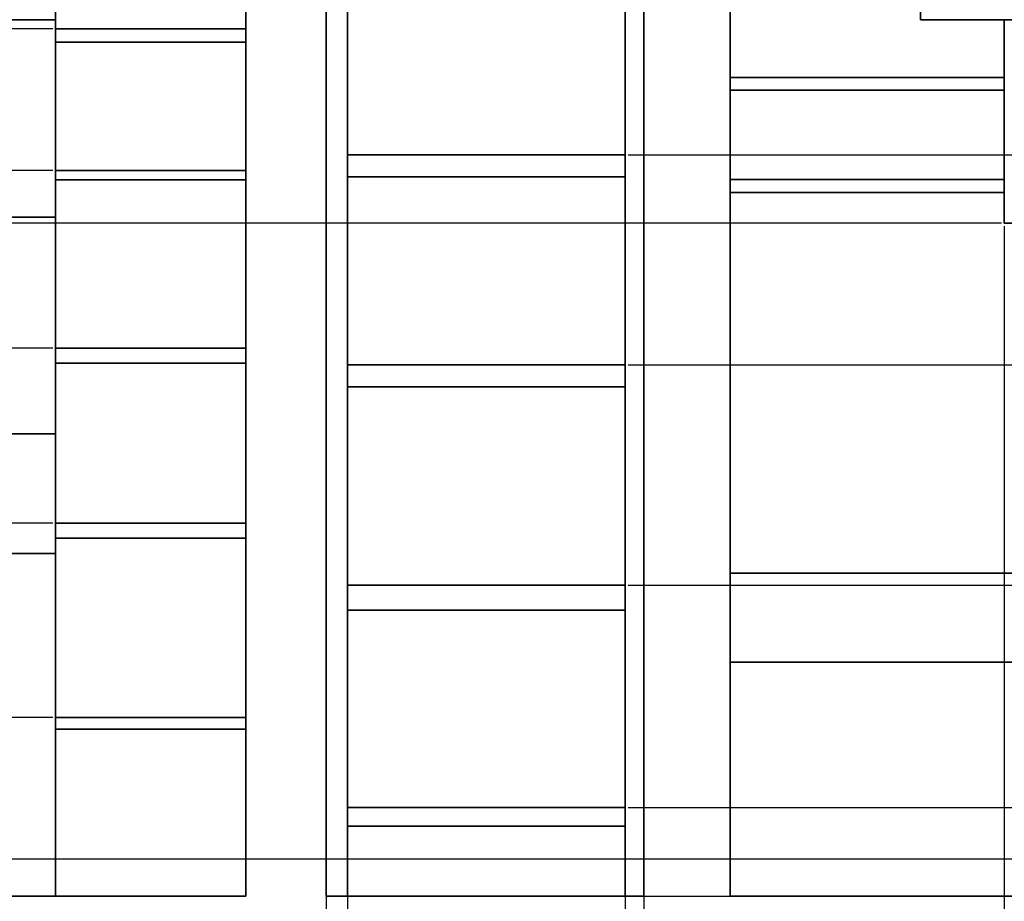
# Model space of a CAD drawing. Units: inches. Extents: x -10 to 130, y -32 to 34.
# Tile 13 of 22: x 49.15 to 70.9, y -13.47 to 6.01. Entities that reach past the tile are written whole.
import ezdxf

# ---------------------------------------------------------------- set-up
doc = ezdxf.new("R2010")
doc.units = ezdxf.units.IN
doc.header["$MEASUREMENT"] = 0
doc.layers.add('A-ANNO-DIMS', color=2, linetype='Continuous', lineweight=18)
doc.layers.add('A-ELEV', color=7, linetype='Continuous', lineweight=35)
doc.styles.get("Standard").update_dxf_attribs({"font": 'arial.ttf'})
doc.dimstyles.get("Standard").update_dxf_attribs({"dimtxt": 0.18, "dimasz": 0.18, "dimexe": 0.18, "dimexo": 0.0625, "dimgap": 0.09, "dimtad": 0, "dimtih": 1, "dimtoh": 1, "dimdec": 4, "dimzin": 0, "dimdsep": 46, "dimtxsty": 'Standard', "dimcen": 0.09, "dimadec": 0, "dimazin": 0, "dimtfac": 1, "dimtdec": 4, "dimtofl": 0, "dimtmove": 0, "dimatfit": 3, "dimfxl": 1, "dimtolj": 1, "dimtzin": 0, "dimarcsym": 0})

# ---------------------------------------------------------------- blocks, each defined once
blk = doc.blocks.new('*D2')
at = {"layer": 'A-ANNO-DIMS', "color": 0, "lineweight": -2, "transparency": 16777216}
for p, q in [((68.738, 27.199), (129.508, 27.199)), ((129.328, 27.019), (129.328, 3.074)), ((129.328, -21.234), (129.328, 2.71)), ((107.996, -21.414), (129.508, -21.414))]:
    blk.add_line(p, q, dxfattribs=at)
at = {"layer": 'A-ANNO-DIMS', "color": 0, "transparency": 16777216}
for points in [[(129.298, 27.019), (129.358, 27.019), (129.328, 27.199)], [(129.298, -21.234), (129.358, -21.234), (129.328, -21.414)]]:
    blk.add_solid(points, dxfattribs=at)
at = {"layer": 'Defpoints', "color": 0, "transparency": 16777216}
for p in [(68.676, 27.199), (129.328, 27.199), (107.933, -21.414)]:
    blk.add_point(p, dxfattribs=at)
at = {"layer": 'A-ANNO-DIMS', "color": 0, "transparency": 16777216, "insert": (129.328, 2.892), "char_height": 0.18, "attachment_point": 5}
blk.add_mtext('\\A1;48.61', dxfattribs=at)
blk = doc.blocks.new('*D33')
at = {"layer": 'A-ANNO-DIMS', "color": 0, "lineweight": -2, "transparency": 16777216}
for p, q in [((70.835, 1.511), (-9.564, 1.511)), ((-9.384, 1.331), (-9.384, 0.73)), ((-9.384, -0.234), (-9.384, 0.367)), ((31.909, -0.414), (-9.564, -0.414))]:
    blk.add_line(p, q, dxfattribs=at)
at = {"layer": 'A-ANNO-DIMS', "color": 0, "transparency": 16777216}
for points in [[(-9.414, 1.331), (-9.354, 1.331), (-9.384, 1.511)], [(-9.414, -0.234), (-9.354, -0.234), (-9.384, -0.414)]]:
    blk.add_solid(points, dxfattribs=at)
at = {"layer": 'Defpoints', "color": 0, "transparency": 16777216}
for p in [(-9.384, 1.511), (70.898, 1.511), (31.971, -0.414)]:
    blk.add_point(p, dxfattribs=at)
at = {"layer": 'A-ANNO-DIMS', "color": 0, "transparency": 16777216, "insert": (-9.384, 0.548), "char_height": 0.18, "attachment_point": 5}
blk.add_mtext('\\A1;1.92', dxfattribs=at)
blk = doc.blocks.new('*D34')
at = {"layer": 'A-ANNO-DIMS', "color": 0, "lineweight": -2, "transparency": 16777216}
for p, q in [((13.34, 6.007), (-9.564, 6.007)), ((-9.384, 5.827), (-9.384, 3.941)), ((-9.384, 1.691), (-9.384, 3.577)), ((70.835, 1.511), (-9.564, 1.511))]:
    blk.add_line(p, q, dxfattribs=at)
at = {"layer": 'A-ANNO-DIMS', "color": 0, "transparency": 16777216}
for points in [[(-9.414, 5.827), (-9.354, 5.827), (-9.384, 6.007)], [(-9.414, 1.691), (-9.354, 1.691), (-9.384, 1.511)]]:
    blk.add_solid(points, dxfattribs=at)
at = {"layer": 'Defpoints', "color": 0, "transparency": 16777216}
for p in [(-9.384, 6.007), (13.402, 6.007), (70.898, 1.511)]:
    blk.add_point(p, dxfattribs=at)
at = {"layer": 'A-ANNO-DIMS', "color": 0, "transparency": 16777216, "insert": (-9.384, 3.759), "char_height": 0.18, "attachment_point": 5}
blk.add_mtext('\\A1;4.497', dxfattribs=at)
blk = doc.blocks.new('*D47')
at = {"layer": 'A-ANNO-DIMS', "color": 0, "lineweight": -2, "transparency": 16777216}
for p, q in [((35.567, -12.534), (129.508, -12.534)), ((129.328, -12.714), (129.328, -16.792)), ((129.328, -21.234), (129.328, -17.156)), ((32.034, -21.414), (129.508, -21.414))]:
    blk.add_line(p, q, dxfattribs=at)
at = {"layer": 'A-ANNO-DIMS', "color": 0, "transparency": 16777216}
for points in [[(129.298, -12.714), (129.358, -12.714), (129.328, -12.534)], [(129.298, -21.234), (129.358, -21.234), (129.328, -21.414)]]:
    blk.add_solid(points, dxfattribs=at)
at = {"layer": 'Defpoints', "color": 0, "transparency": 16777216}
for p in [(35.505, -12.534), (31.971, -21.414), (129.328, -21.414)]:
    blk.add_point(p, dxfattribs=at)
at = {"layer": 'A-ANNO-DIMS', "color": 0, "transparency": 16777216, "insert": (129.328, -16.974), "char_height": 0.18, "attachment_point": 5}
blk.add_mtext('\\A1;8.88', dxfattribs=at)
blk = doc.blocks.new('*D48')
at = {"layer": 'A-ANNO-DIMS', "color": 0, "lineweight": -2, "transparency": 16777216}
for p, q in [((44.76, -13.293), (44.76, 33.879)), ((74.492, -13.293), (74.492, 33.879)), ((44.94, 33.699), (59.231, 33.699)), ((74.312, 33.699), (60.021, 33.699))]:
    blk.add_line(p, q, dxfattribs=at)
at = {"layer": 'A-ANNO-DIMS', "color": 0, "transparency": 16777216}
for points in [[(44.94, 33.729), (44.94, 33.669), (44.76, 33.699)], [(74.312, 33.729), (74.312, 33.669), (74.492, 33.699)]]:
    blk.add_solid(points, dxfattribs=at)
at = {"layer": 'Defpoints', "color": 0, "transparency": 16777216}
for p in [(74.492, 33.699), (44.76, -13.356), (74.492, -13.356)]:
    blk.add_point(p, dxfattribs=at)
at = {"layer": 'A-ANNO-DIMS', "color": 0, "transparency": 16777216, "insert": (59.626, 33.699), "char_height": 0.18, "attachment_point": 5}
blk.add_mtext('\\A1;29.73', dxfattribs=at)
blk = doc.blocks.new('*D72')
at = {"layer": 'A-ANNO-DIMS', "color": 0, "lineweight": -2, "transparency": 16777216}
for p, q in [((55.918, 16.529), (55.918, -28.129)), ((62.934, 16.482), (62.934, -28.129)), ((56.098, -27.949), (59.033, -27.949)), ((62.754, -27.949), (59.819, -27.949))]:
    blk.add_line(p, q, dxfattribs=at)
at = {"layer": 'A-ANNO-DIMS', "color": 0, "transparency": 16777216}
for points in [[(56.098, -27.919), (56.098, -27.979), (55.918, -27.949)], [(62.754, -27.919), (62.754, -27.979), (62.934, -27.949)]]:
    blk.add_solid(points, dxfattribs=at)
at = {"layer": 'Defpoints', "color": 0, "transparency": 16777216}
for p in [(55.918, 16.591), (62.934, 16.545), (62.934, -27.949)]:
    blk.add_point(p, dxfattribs=at)
at = {"layer": 'A-ANNO-DIMS', "color": 0, "transparency": 16777216, "insert": (59.426, -27.949), "char_height": 0.18, "attachment_point": 5}
blk.add_mtext('\\A1;7.016', dxfattribs=at)
blk = doc.blocks.new('*D73')
at = {"layer": 'A-ANNO-DIMS', "color": 0, "lineweight": -2, "transparency": 16777216}
for p, q in [((56.395, 16.255), (56.395, -28.129)), ((62.526, 16.255), (62.526, -28.129)), ((56.575, -27.949), (59.083, -27.949)), ((62.346, -27.949), (59.837, -27.949))]:
    blk.add_line(p, q, dxfattribs=at)
at = {"layer": 'A-ANNO-DIMS', "color": 0, "transparency": 16777216}
for points in [[(56.575, -27.919), (56.575, -27.979), (56.395, -27.949)], [(62.346, -27.919), (62.346, -27.979), (62.526, -27.949)]]:
    blk.add_solid(points, dxfattribs=at)
at = {"layer": 'Defpoints', "color": 0, "transparency": 16777216}
for p in [(56.395, 16.317), (62.526, 16.317), (62.526, -27.949)]:
    blk.add_point(p, dxfattribs=at)
at = {"layer": 'A-ANNO-DIMS', "color": 0, "transparency": 16777216, "insert": (59.46, -27.949), "char_height": 0.18, "attachment_point": 5}
blk.add_mtext('\\A1;6.131', dxfattribs=at)
blk = doc.blocks.new('*D75')
at = {"layer": 'A-ANNO-DIMS', "color": 0, "lineweight": -2, "transparency": 16777216}
for p, q in [((62.588, -11.398), (129.508, -11.398)), ((129.328, -11.578), (129.328, -12.195)), ((129.328, -13.176), (129.328, -12.559)), ((62.588, -13.356), (129.508, -13.356))]:
    blk.add_line(p, q, dxfattribs=at)
at = {"layer": 'A-ANNO-DIMS', "color": 0, "transparency": 16777216}
for points in [[(129.298, -11.578), (129.358, -11.578), (129.328, -11.398)], [(129.298, -13.176), (129.358, -13.176), (129.328, -13.356)]]:
    blk.add_solid(points, dxfattribs=at)
at = {"layer": 'Defpoints', "color": 0, "transparency": 16777216}
for p in [(62.526, -11.398), (129.328, -11.398), (62.526, -13.356)]:
    blk.add_point(p, dxfattribs=at)
at = {"layer": 'A-ANNO-DIMS', "color": 0, "transparency": 16777216, "insert": (129.328, -12.377), "char_height": 0.18, "attachment_point": 5}
blk.add_mtext('\\A1;1.96', dxfattribs=at)
blk = doc.blocks.new('*D76')
at = {"layer": 'A-ANNO-DIMS', "color": 0, "lineweight": -2, "transparency": 16777216}
for p, q in [((62.588, -6.485), (129.508, -6.485)), ((129.328, -6.665), (129.328, -8.76)), ((129.328, -11.218), (129.328, -9.123)), ((62.588, -11.398), (129.508, -11.398))]:
    blk.add_line(p, q, dxfattribs=at)
at = {"layer": 'A-ANNO-DIMS', "color": 0, "transparency": 16777216}
for points in [[(129.298, -6.665), (129.358, -6.665), (129.328, -6.485)], [(129.298, -11.218), (129.358, -11.218), (129.328, -11.398)]]:
    blk.add_solid(points, dxfattribs=at)
at = {"layer": 'Defpoints', "color": 0, "transparency": 16777216}
for p in [(62.526, -6.485), (129.328, -6.485), (62.526, -11.398)]:
    blk.add_point(p, dxfattribs=at)
at = {"layer": 'A-ANNO-DIMS', "color": 0, "transparency": 16777216, "insert": (129.328, -8.942), "char_height": 0.18, "attachment_point": 5}
blk.add_mtext('\\A1;4.913', dxfattribs=at)
blk = doc.blocks.new('*D77')
at = {"layer": 'A-ANNO-DIMS', "color": 0, "lineweight": -2, "transparency": 16777216}
for p, q in [((62.588, -1.618), (129.508, -1.618)), ((129.328, -1.798), (129.328, -3.87)), ((129.328, -6.305), (129.328, -4.234)), ((62.588, -6.485), (129.508, -6.485))]:
    blk.add_line(p, q, dxfattribs=at)
at = {"layer": 'A-ANNO-DIMS', "color": 0, "transparency": 16777216}
for points in [[(129.298, -1.798), (129.358, -1.798), (129.328, -1.618)], [(129.298, -6.305), (129.358, -6.305), (129.328, -6.485)]]:
    blk.add_solid(points, dxfattribs=at)
at = {"layer": 'Defpoints', "color": 0, "transparency": 16777216}
for p in [(62.526, -1.618), (129.328, -1.618), (62.526, -6.485)]:
    blk.add_point(p, dxfattribs=at)
at = {"layer": 'A-ANNO-DIMS', "color": 0, "transparency": 16777216, "insert": (129.328, -4.052), "char_height": 0.18, "attachment_point": 5}
blk.add_mtext('\\A1;4.866', dxfattribs=at)
blk = doc.blocks.new('*D78')
at = {"layer": 'A-ANNO-DIMS', "color": 0, "lineweight": -2, "transparency": 16777216}
for p, q in [((62.588, 3.018), (129.508, 3.018)), ((129.328, 2.838), (129.328, 0.882)), ((129.328, -1.438), (129.328, 0.518)), ((62.588, -1.618), (129.508, -1.618))]:
    blk.add_line(p, q, dxfattribs=at)
at = {"layer": 'A-ANNO-DIMS', "color": 0, "transparency": 16777216}
for points in [[(129.298, 2.838), (129.358, 2.838), (129.328, 3.018)], [(129.298, -1.438), (129.358, -1.438), (129.328, -1.618)]]:
    blk.add_solid(points, dxfattribs=at)
at = {"layer": 'Defpoints', "color": 0, "transparency": 16777216}
for p in [(62.526, 3.018), (129.328, 3.018), (62.526, -1.618)]:
    blk.add_point(p, dxfattribs=at)
at = {"layer": 'A-ANNO-DIMS', "color": 0, "transparency": 16777216, "insert": (129.328, 0.7), "char_height": 0.18, "attachment_point": 5}
blk.add_mtext('\\A1;4.64', dxfattribs=at)
blk = doc.blocks.new('*D79')
at = {"layer": 'A-ANNO-DIMS', "color": 0, "lineweight": -2, "transparency": 16777216}
for p, q in [((62.588, 7.736), (129.508, 7.736)), ((129.328, 7.556), (129.328, 5.559)), ((129.328, 3.198), (129.328, 5.195)), ((62.588, 3.018), (129.508, 3.018))]:
    blk.add_line(p, q, dxfattribs=at)
at = {"layer": 'A-ANNO-DIMS', "color": 0, "transparency": 16777216}
for points in [[(129.298, 7.556), (129.358, 7.556), (129.328, 7.736)], [(129.298, 3.198), (129.358, 3.198), (129.328, 3.018)]]:
    blk.add_solid(points, dxfattribs=at)
at = {"layer": 'Defpoints', "color": 0, "transparency": 16777216}
for p in [(62.526, 7.736), (129.328, 7.736), (62.526, 3.018)]:
    blk.add_point(p, dxfattribs=at)
at = {"layer": 'A-ANNO-DIMS', "color": 0, "transparency": 16777216, "insert": (129.328, 5.377), "char_height": 0.18, "attachment_point": 5}
blk.add_mtext('\\A1;4.718', dxfattribs=at)
blk = doc.blocks.new('*D89')
at = {"layer": 'A-ANNO-DIMS', "color": 0, "lineweight": -2, "transparency": 16777216}
for p, q in [((49.884, 9.058), (-9.564, 9.058)), ((-9.384, 8.878), (-9.384, 7.612)), ((-9.384, 5.982), (-9.384, 7.248)), ((49.884, 5.802), (-9.564, 5.802))]:
    blk.add_line(p, q, dxfattribs=at)
at = {"layer": 'A-ANNO-DIMS', "color": 0, "transparency": 16777216}
for points in [[(-9.414, 8.878), (-9.354, 8.878), (-9.384, 9.058)], [(-9.414, 5.982), (-9.354, 5.982), (-9.384, 5.802)]]:
    blk.add_solid(points, dxfattribs=at)
at = {"layer": 'Defpoints', "color": 0, "transparency": 16777216}
for p in [(49.946, 9.058), (-9.384, 5.802), (49.946, 5.802)]:
    blk.add_point(p, dxfattribs=at)
at = {"layer": 'A-ANNO-DIMS', "color": 0, "transparency": 16777216, "insert": (-9.384, 7.43), "char_height": 0.18, "attachment_point": 5}
blk.add_mtext('\\A1;3.256', dxfattribs=at)
blk = doc.blocks.new('*D90')
at = {"layer": 'A-ANNO-DIMS', "color": 0, "lineweight": -2, "transparency": 16777216}
for p, q in [((49.884, 5.802), (-9.564, 5.802)), ((-9.384, 5.622), (-9.384, 4.421)), ((-9.384, 2.855), (-9.384, 4.057)), ((49.884, 2.675), (-9.564, 2.675))]:
    blk.add_line(p, q, dxfattribs=at)
at = {"layer": 'A-ANNO-DIMS', "color": 0, "transparency": 16777216}
for points in [[(-9.414, 5.622), (-9.354, 5.622), (-9.384, 5.802)], [(-9.414, 2.855), (-9.354, 2.855), (-9.384, 2.675)]]:
    blk.add_solid(points, dxfattribs=at)
at = {"layer": 'Defpoints', "color": 0, "transparency": 16777216}
for p in [(49.946, 5.802), (-9.384, 2.675), (49.946, 2.675)]:
    blk.add_point(p, dxfattribs=at)
at = {"layer": 'A-ANNO-DIMS', "color": 0, "transparency": 16777216, "insert": (-9.384, 4.239), "char_height": 0.18, "attachment_point": 5}
blk.add_mtext('\\A1;3.127', dxfattribs=at)
blk = doc.blocks.new('*D91')
at = {"layer": 'A-ANNO-DIMS', "color": 0, "lineweight": -2, "transparency": 16777216}
for p, q in [((49.884, 2.675), (-9.564, 2.675)), ((-9.384, 2.495), (-9.384, 0.895)), ((-9.384, -1.07), (-9.384, 0.531)), ((49.884, -1.25), (-9.564, -1.25))]:
    blk.add_line(p, q, dxfattribs=at)
at = {"layer": 'A-ANNO-DIMS', "color": 0, "transparency": 16777216}
for points in [[(-9.414, 2.495), (-9.354, 2.495), (-9.384, 2.675)], [(-9.414, -1.07), (-9.354, -1.07), (-9.384, -1.25)]]:
    blk.add_solid(points, dxfattribs=at)
at = {"layer": 'Defpoints', "color": 0, "transparency": 16777216}
for p in [(49.946, 2.675), (-9.384, -1.25), (49.946, -1.25)]:
    blk.add_point(p, dxfattribs=at)
at = {"layer": 'A-ANNO-DIMS', "color": 0, "transparency": 16777216, "insert": (-9.384, 0.713), "char_height": 0.18, "attachment_point": 5}
blk.add_mtext('\\A1;3.925', dxfattribs=at)
blk = doc.blocks.new('*D92')
at = {"layer": 'A-ANNO-DIMS', "color": 0, "lineweight": -2, "transparency": 16777216}
for p, q in [((49.884, -1.25), (-9.564, -1.25)), ((-9.384, -1.43), (-9.384, -3.001)), ((-9.384, -4.936), (-9.384, -3.365)), ((49.884, -5.116), (-9.564, -5.116))]:
    blk.add_line(p, q, dxfattribs=at)
at = {"layer": 'A-ANNO-DIMS', "color": 0, "transparency": 16777216}
for points in [[(-9.414, -1.43), (-9.354, -1.43), (-9.384, -1.25)], [(-9.414, -4.936), (-9.354, -4.936), (-9.384, -5.116)]]:
    blk.add_solid(points, dxfattribs=at)
at = {"layer": 'Defpoints', "color": 0, "transparency": 16777216}
for p in [(49.946, -1.25), (-9.384, -5.116), (49.946, -5.116)]:
    blk.add_point(p, dxfattribs=at)
at = {"layer": 'A-ANNO-DIMS', "color": 0, "transparency": 16777216, "insert": (-9.384, -3.183), "char_height": 0.18, "attachment_point": 5}
blk.add_mtext('\\A1;3.866', dxfattribs=at)
blk = doc.blocks.new('*D93')
at = {"layer": 'A-ANNO-DIMS', "color": 0, "lineweight": -2, "transparency": 16777216}
for p, q in [((49.884, -5.116), (-9.564, -5.116)), ((-9.384, -5.296), (-9.384, -7.081)), ((-9.384, -9.23), (-9.384, -7.445)), ((49.884, -9.41), (-9.564, -9.41))]:
    blk.add_line(p, q, dxfattribs=at)
at = {"layer": 'A-ANNO-DIMS', "color": 0, "transparency": 16777216}
for points in [[(-9.414, -5.296), (-9.354, -5.296), (-9.384, -5.116)], [(-9.414, -9.23), (-9.354, -9.23), (-9.384, -9.41)]]:
    blk.add_solid(points, dxfattribs=at)
at = {"layer": 'Defpoints', "color": 0, "transparency": 16777216}
for p in [(49.946, -5.116), (-9.384, -9.41), (49.946, -9.41)]:
    blk.add_point(p, dxfattribs=at)
at = {"layer": 'A-ANNO-DIMS', "color": 0, "transparency": 16777216, "insert": (-9.384, -7.263), "char_height": 0.18, "attachment_point": 5}
blk.add_mtext('\\A1;4.294', dxfattribs=at)
blk = doc.blocks.new('*D94')
at = {"layer": 'A-ANNO-DIMS', "color": 0, "lineweight": -2, "transparency": 16777216}
for p, q in [((49.884, -9.41), (-9.564, -9.41)), ((-9.384, -9.59), (-9.384, -11.201)), ((-9.384, -13.176), (-9.384, -11.565)), ((49.884, -13.356), (-9.564, -13.356))]:
    blk.add_line(p, q, dxfattribs=at)
at = {"layer": 'A-ANNO-DIMS', "color": 0, "transparency": 16777216}
for points in [[(-9.414, -9.59), (-9.354, -9.59), (-9.384, -9.41)], [(-9.414, -13.176), (-9.354, -13.176), (-9.384, -13.356)]]:
    blk.add_solid(points, dxfattribs=at)
at = {"layer": 'Defpoints', "color": 0, "transparency": 16777216}
for p in [(49.946, -9.41), (-9.384, -13.356), (49.946, -13.356)]:
    blk.add_point(p, dxfattribs=at)
at = {"layer": 'A-ANNO-DIMS', "color": 0, "transparency": 16777216, "insert": (-9.384, -11.383), "char_height": 0.18, "attachment_point": 5}
blk.add_mtext('\\A1;3.946', dxfattribs=at)
blk = doc.blocks.new('*D139')
at = {"layer": 'A-ANNO-DIMS', "color": 0, "lineweight": -2, "transparency": 16777216}
for p, q in [((70.057, 6.643), (129.508, 6.643)), ((129.328, 6.463), (129.328, 6.187)), ((69.108, 6.007), (129.508, 6.007)), ((129.328, 6.007), (129.328, 5.827)), ((129.328, 5.827), (129.148, 5.827))]:
    blk.add_line(p, q, dxfattribs=at)
at = {"layer": 'A-ANNO-DIMS', "color": 0, "transparency": 16777216}
for points in [[(129.298, 6.463), (129.358, 6.463), (129.328, 6.643)], [(129.298, 6.187), (129.358, 6.187), (129.328, 6.007)]]:
    blk.add_solid(points, dxfattribs=at)
at = {"layer": 'Defpoints', "color": 0, "transparency": 16777216}
for p in [(69.995, 6.643), (69.045, 6.007), (129.328, 6.007)]:
    blk.add_point(p, dxfattribs=at)
at = {"layer": 'A-ANNO-DIMS', "color": 0, "transparency": 16777216, "insert": (128.754, 5.827), "char_height": 0.18, "attachment_point": 5}
blk.add_mtext('\\A1;0.636', dxfattribs=at)
blk = doc.blocks.new('*D155')
at = {"layer": 'A-ANNO-DIMS', "color": 0, "lineweight": -2, "transparency": 16777216}
for p, q in [((70.897993, 1.448166), (70.897993, -28.129305)), ((71.936707, 1.448166), (71.936707, -28.129305)), ((70.717993, -27.949305), (70.537993, -27.949305)), ((72.116707, -27.949305), (72.296707, -27.949305))]:
    blk.add_line(p, q, dxfattribs=at)
at = {"layer": 'A-ANNO-DIMS', "color": 0, "transparency": 16777216}
for points in [[(70.717993, -27.919305), (70.717993, -27.979305), (70.897993, -27.949305)], [(72.116707, -27.919305), (72.116707, -27.979305), (71.936707, -27.949305)]]:
    blk.add_solid(points, dxfattribs=at)
at = {"layer": 'Defpoints', "color": 0, "transparency": 16777216}
for p in [(70.897993, 1.510666), (71.936707, 1.510666), (71.936707, -27.949305)]:
    blk.add_point(p, dxfattribs=at)
at = {"layer": 'A-ANNO-DIMS', "color": 0, "transparency": 16777216, "insert": (71.41735, -27.949305), "char_height": 0.18, "attachment_point": 5}
blk.add_mtext('\\A1;1.039', dxfattribs=at)

msp = doc.modelspace()

# ---------------------------------------------------------------- linework, layer by layer
at = {"layer": 'A-ELEV'}
for p, q in [((54.1471, 17.6074), (54.1471, -13.3558)), ((64.8443, 17.6074), (64.8443, -13.3558)), ((55.9182, 16.5911), (55.9182, -13.3558)), ((62.9343, 16.5448), (62.9343, -13.3558)), ((56.395, 16.3174), (56.395, -13.3558)), ((62.5256, 16.3174), (62.5256, -13.3558)), ((49.9462, 6.0074), (49.9462, 14.8409)), ((69.0452, 6.0074), (69.0452, 14.8409)), ((20.3124, 6.0074), (49.9462, 6.0074)), ((49.9462, 6.0074), (49.9462, -13.3558)), ((98.6791, 6.0074), (69.0452, 6.0074)), ((70.898, 6.0074), (70.898, 1.5107)), ((49.9462, 5.8024), (54.1471, 5.8024)), ((49.9462, 5.5072), (54.1471, 5.5072)), ((70.898, 4.7338), (64.8443, 4.7338)), ((70.898, 4.4512), (64.8443, 4.4512)), ((56.395, 3.0181), (62.5256, 3.0181)), ((49.9462, 2.6753), (54.1471, 2.6753)), ((49.9462, 2.4695), (54.1471, 2.4695)), ((56.395, 2.5337), (62.5256, 2.5337)), ((70.898, 2.4733), (64.8443, 2.4733)), ((70.898, 2.1908), (64.8443, 2.1908)), ((46.4227, 1.6419), (49.9462, 1.6419)), ((70.898, 1.5107), (81.4053, 1.5107)), ((49.9462, -1.2496), (54.1471, -1.2496)), ((49.9462, -1.5799), (54.1471, -1.5799)), ((56.395, -1.6184), (62.5256, -1.6184)), ((56.395, -2.1028), (62.5256, -2.1028)), ((42.7881, -3.1438), (49.9462, -3.1438)), ((49.9462, -5.1155), (54.1471, -5.1155)), ((49.9462, -5.4458), (54.1471, -5.4458)), ((46.8089, -5.7836), (49.9462, -5.7836)), ((71.9367, -6.2218), (64.8443, -6.2218)), ((56.395, -6.4849), (62.5256, -6.4849)), ((56.395, -7.0385), (62.5256, -7.0385)), ((71.9367, -8.1891), (64.8443, -8.1891)), ((49.9462, -9.4098), (54.1471, -9.4098)), ((49.9462, -9.6667), (54.1471, -9.6667)), ((56.395, -11.3982), (62.5256, -11.3982)), ((56.395, -11.8134), (62.5256, -11.8134)), ((54.1471, -13.3558), (44.76, -13.3558)), ((55.9182, -13.3558), (62.9343, -13.3558)), ((64.8443, -13.3558), (74.492, -13.3558))]:
    msp.add_line(p, q, dxfattribs=at)

# ---------------------------------------------------------------- dimensions: what is measured, and where the dimension line sits
at = {"layer": 'A-ANNO-DIMS'}
for base, p1, p2, override, picture, middle in [((74.492, 33.6987), (44.76, -13.3558), (74.492, -13.3558), {"dimdec": 2, "dimlfac": 1, "dimrnd": 0, "dimzin": 0, "dimdsep": 46, "dimlunit": 2}, '*D48', (59.626, 33.6987)), ((62.9343, -27.9493), (55.9182, 16.5911), (62.9343, 16.5448), {"dimdec": 3, "dimlfac": 1, "dimrnd": 0, "dimzin": 0, "dimdsep": 46, "dimlunit": 2}, '*D72', (59.4263, -27.9493)), ((62.5256, -27.9493), (56.395, 16.3174), (62.5256, 16.3174), {"dimdec": 3, "dimlfac": 1, "dimrnd": 0, "dimzin": 0, "dimdsep": 46, "dimlunit": 2}, '*D73', (59.4603, -27.9493)), ((71.9367, -27.9493), (70.898, 1.5107), (71.9367, 1.5107), {"dimdec": 3, "dimlfac": 1, "dimrnd": 0, "dimzin": 0, "dimdsep": 46, "dimlunit": 2}, '*D155', (71.4173, -27.9493))]:
    dim = msp.add_linear_dim(base=base, p1=p1, p2=p2, dimstyle='Standard', override=override, dxfattribs=at)
    dim.commit()
    dim.dimension.update_dxf_attribs({"geometry": picture, "text_midpoint": middle})
for base, p1, p2, override, picture, middle in [((129.3277, 27.1987), (107.9333, -21.4145), (68.6759, 27.1987), {"dimdec": 2, "dimlfac": 1, "dimrnd": 0, "dimzin": 0, "dimdsep": 46, "dimlunit": 2}, '*D2', (129.3277, 2.8921)), ((-9.3836, 5.8024), (49.9462, 9.058), (49.9462, 5.8024), {"dimdec": 3, "dimlfac": 1, "dimrnd": 0, "dimzin": 0, "dimdsep": 46, "dimlunit": 2}, '*D89', (-9.3836, 7.4302)), ((129.3277, 7.7364), (62.5256, 3.0181), (62.5256, 7.7364), {"dimdec": 3, "dimlfac": 1, "dimrnd": 0, "dimzin": 0, "dimdsep": 46, "dimlunit": 2}, '*D79', (129.3277, 5.3773)), ((129.3277, 6.0074), (69.9946, 6.6433), (69.0452, 6.0074), {"dimdec": 3, "dimlfac": 1, "dimrnd": 0, "dimzin": 0, "dimdsep": 46, "dimlunit": 2}, '*D139', (128.754, 5.8274)), ((-9.3836, 6.0074), (70.898, 1.5107), (13.4021, 6.0074), {"dimdec": 3, "dimlfac": 1, "dimrnd": 0, "dimzin": 0, "dimdsep": 46, "dimlunit": 2}, '*D34', (-9.3836, 3.7591)), ((-9.3836, 2.6753), (49.9462, 5.8024), (49.9462, 2.6753), {"dimdec": 3, "dimlfac": 1, "dimrnd": 0, "dimzin": 0, "dimdsep": 46, "dimlunit": 2}, '*D90', (-9.3836, 4.2388)), ((129.3277, 3.0181), (62.5256, -1.6184), (62.5256, 3.0181), {"dimdec": 2, "dimlfac": 1, "dimrnd": 0, "dimzin": 0, "dimdsep": 46, "dimlunit": 2}, '*D78', (129.3277, 0.6998)), ((-9.3836, -1.2496), (49.9462, 2.6753), (49.9462, -1.2496), {"dimdec": 3, "dimlfac": 1, "dimrnd": 0, "dimzin": 0, "dimdsep": 46, "dimlunit": 2}, '*D91', (-9.3836, 0.7128)), ((-9.3836, 1.5107), (31.9712, -0.4138), (70.898, 1.5107), {"dimdec": 2, "dimlfac": 1, "dimrnd": 0, "dimzin": 0, "dimdsep": 46, "dimlunit": 2}, '*D33', (-9.3836, 0.5484)), ((-9.3836, -5.1155), (49.9462, -1.2496), (49.9462, -5.1155), {"dimdec": 3, "dimlfac": 1, "dimrnd": 0, "dimzin": 0, "dimdsep": 46, "dimlunit": 2}, '*D92', (-9.3836, -3.1826)), ((129.32767, -1.61843), (62.52563, -6.48486), (62.52563, -1.61843), {"dimdec": 3, "dimlfac": 1, "dimrnd": 0, "dimzin": 0, "dimdsep": 46, "dimlunit": 2}, '*D77', (129.32767, -4.05165)), ((-9.3836, -9.4098), (49.9462, -5.1155), (49.9462, -9.4098), {"dimdec": 3, "dimlfac": 1, "dimrnd": 0, "dimzin": 0, "dimdsep": 46, "dimlunit": 2}, '*D93', (-9.3836, -7.2626)), ((129.3277, -6.4849), (62.5256, -11.3982), (62.5256, -6.4849), {"dimdec": 3, "dimlfac": 1, "dimrnd": 0, "dimzin": 0, "dimdsep": 46, "dimlunit": 2}, '*D76', (129.3277, -8.9415)), ((-9.3836, -13.3558), (49.9462, -9.4098), (49.9462, -13.3558), {"dimdec": 3, "dimlfac": 1, "dimrnd": 0, "dimzin": 0, "dimdsep": 46, "dimlunit": 2}, '*D94', (-9.3836, -11.3828)), ((129.3277, -11.3982), (62.5256, -13.3558), (62.5256, -11.3982), {"dimdec": 2, "dimlfac": 1, "dimrnd": 0, "dimzin": 0, "dimdsep": 46, "dimlunit": 2}, '*D75', (129.3277, -12.377)), ((129.3277, -21.4145), (35.5046, -12.5339), (31.9712, -21.4145), {"dimdec": 2, "dimlfac": 1, "dimrnd": 0, "dimzin": 0, "dimdsep": 46, "dimlunit": 2}, '*D47', (129.3277, -16.9742))]:
    dim = msp.add_linear_dim(base=base, p1=p1, p2=p2, angle=90, dimstyle='Standard', override=override, dxfattribs=at)
    dim.commit()
    dim.dimension.update_dxf_attribs({"geometry": picture, "text_midpoint": middle})

doc.saveas('drawing.dxf')
